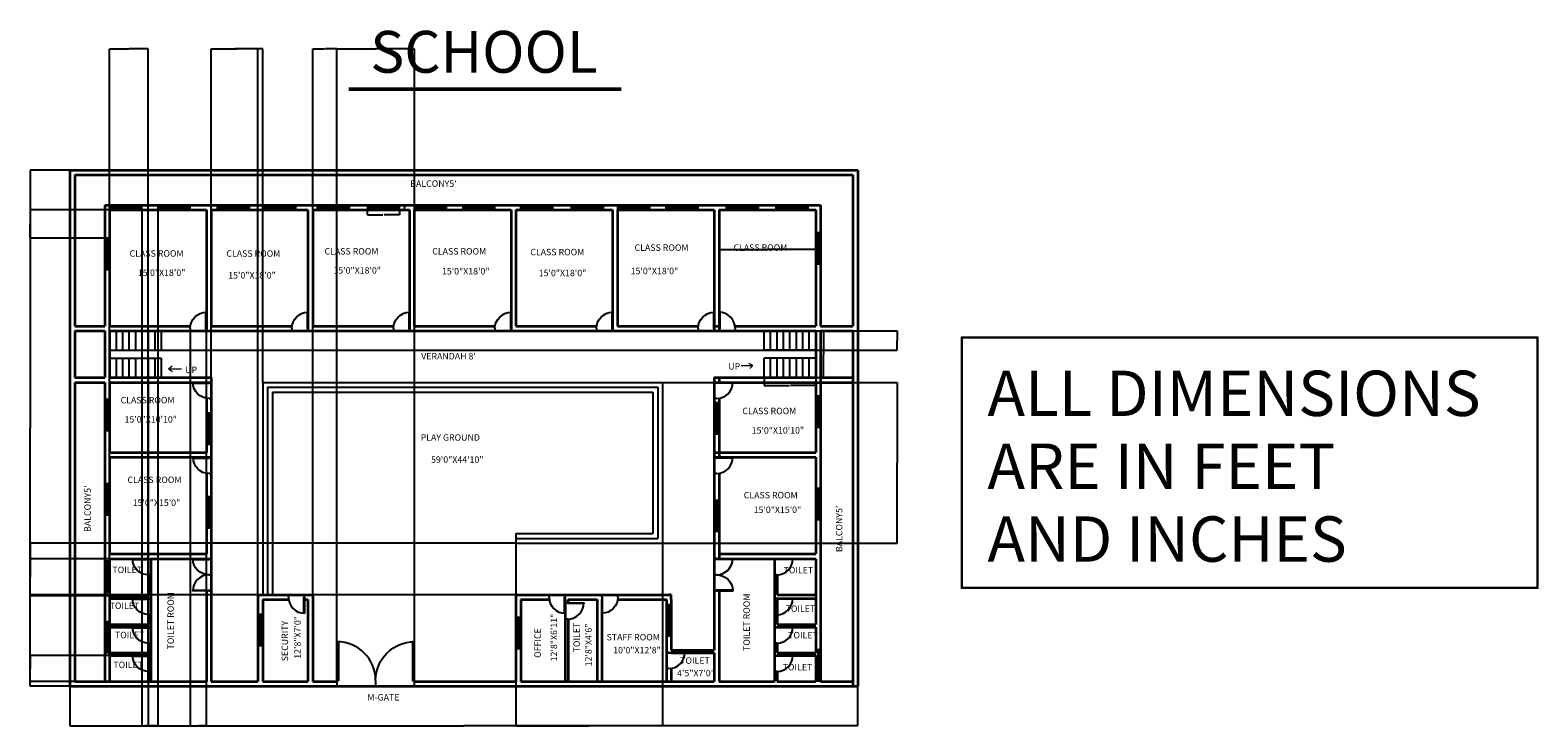
# Model space of a CAD drawing. Units: inches. Extents: x 232314 to 235120, y 482029 to 483323.
import ezdxf

# ---------------------------------------------------------------- set-up
doc = ezdxf.new("R2010")
doc.units = ezdxf.units.IN
for name, color, linetype, lineweight in [('A-ANNO-DIMS', 3, 'Continuous', 18), ('A-ANNO-SYMB', 7, 'Continuous', 18), ('A-ANNO-TEXT', 7, 'Continuous', 18), ('A-ANNO-TTLB', 6, 'Continuous', 35), ('A-AREA-IDEN', 3, 'Continuous', 18), ('A-FLOR-EDGE', 7, 'Continuous', 25), ('A-FLOR-STRS', 7, 'Continuous', 25), ('A-GLAZ', 5, 'Continuous', 18), ('A-WALL', 7, 'Continuous', 35), ('doors', 4, 'Continuous', 25)]:
    doc.layers.add(name, color=color, linetype=linetype, lineweight=lineweight)
doc.styles.get("Standard").update_dxf_attribs({"font": 'arial.ttf'})
doc.dimstyles.get("Standard").update_dxf_attribs({"dimtxt": 0.18, "dimasz": 0.18, "dimexe": 0.18, "dimexo": 0.0625, "dimgap": 0.09, "dimtad": 0, "dimtih": 1, "dimtoh": 1, "dimdec": 4, "dimzin": 0, "dimdsep": 46, "dimtxsty": 'Standard', "dimcen": 0.09, "dimadec": 0, "dimazin": 0, "dimtfac": 1, "dimtdec": 4, "dimtofl": 0, "dimtmove": 0, "dimatfit": 3, "dimfxl": 1, "dimtolj": 1, "dimtzin": 0, "dimarcsym": 0})

# ---------------------------------------------------------------- blocks, each defined once
blk = doc.blocks.new('*U2')
for p, q in [((0, 0), (0, -6)), ((40, 0), (40, -6))]:
    blk.add_line(p, q)
blk.add_lwpolyline([(0, 0), (0, 40), (1.75, 40), (1.75, 0)], close=True)
blk.add_arc((0, 0), 40, 0, 90)
blk = doc.blocks.new('WIN-60X9-IN')
for p, q in [((0, 5.5), (60, 5.5)), ((0, 3.5), (60, 3.5))]:
    blk.add_line(p, q)
blk.add_lwpolyline([(0, 9), (60, 9), (60, 0), (0, 0)], close=True)
blk = doc.blocks.new('STAIR-PAIRED-FLIGHT')
for p, q in [((12, 87), (12, 51)), ((24, 87), (24, 51)), ((36, 87), (36, 51)), ((48, 87), (48, 51)), ((60, 87), (60, 51)), ((72, 87), (72, 51)), ((84, 87), (84, 51)), ((96, 87), (96, 51)), ((0, 51), (96, 51)), ((0, 36), (96, 36)), ((12, 36), (12, 0)), ((24, 36), (24, 0)), ((36, 36), (36, 0)), ((48, 36), (48, 0)), ((60, 36), (60, 0)), ((72, 36), (72, 0)), ((84, 36), (84, 0)), ((96, 36), (96, 0))]:
    blk.add_line(p, q)
blk = doc.blocks.new('*D7')
at = {"layer": 'A-ANNO-DIMS', "color": 0, "lineweight": -2, "transparency": 16777216}
for p, q in [((232941.9, 482988.3), (232941.9, 482979.2)), ((232942.1, 482979.4), (232970.8, 482979.4)), ((233001.7, 482979.4), (232973, 482979.4)), ((233001.9, 482988.3), (233001.9, 482979.2))]:
    blk.add_line(p, q, dxfattribs=at)
at = {"layer": 'A-ANNO-DIMS', "color": 0, "transparency": 16777216}
for points in [[(232942.1, 482979.4), (232942.1, 482979.3), (232941.9, 482979.4)], [(233001.7, 482979.4), (233001.7, 482979.3), (233001.9, 482979.4)]]:
    blk.add_solid(points, dxfattribs=at)
at = {"layer": 'Defpoints', "color": 0, "transparency": 16777216}
for p in [(232941.9, 482988.4), (233001.9, 482988.4), (233001.9, 482979.4)]:
    blk.add_point(p, dxfattribs=at)
at = {"layer": 'A-ANNO-DIMS', "color": 0, "transparency": 16777216, "insert": (232971.9, 482979.4), "char_height": 0.18, "attachment_point": 5}
blk.add_mtext('\\A1;WINDOW 60 TYP.', dxfattribs=at)
blk = doc.blocks.new('*D8')
at = {"layer": 'A-ANNO-DIMS', "color": 0, "lineweight": -2, "transparency": 16777216}
for p, q in [((233002, 482997.4), (233011.1, 482997.4)), ((233002, 482988.4), (233011.1, 482988.4)), ((233010.9, 482997.2), (233010.9, 482993.1)), ((233010.9, 482988.6), (233010.9, 482992.7))]:
    blk.add_line(p, q, dxfattribs=at)
at = {"layer": 'A-ANNO-DIMS', "color": 0, "transparency": 16777216}
for points in [[(233010.9, 482997.2), (233011, 482997.2), (233010.9, 482997.4)], [(233010.9, 482988.6), (233011, 482988.6), (233010.9, 482988.4)]]:
    blk.add_solid(points, dxfattribs=at)
at = {"layer": 'Defpoints', "color": 0, "transparency": 16777216}
for p in [(233001.9, 482997.4), (233001.9, 482988.4), (233010.9, 482997.4)]:
    blk.add_point(p, dxfattribs=at)
at = {"layer": 'A-ANNO-DIMS', "color": 0, "transparency": 16777216, "insert": (233010.9, 482992.9), "char_height": 0.18, "attachment_point": 5}
blk.add_mtext('\\A1;9 TYP.', dxfattribs=at)
blk = doc.blocks.new('*D9')
at = {"layer": 'A-ANNO-DIMS', "color": 0, "lineweight": -2, "transparency": 16777216}
for p, q in [((233680.3, 482676.3), (233680.3, 482661.8)), ((233776.3, 482676.3), (233776.3, 482661.8)), ((233680.5, 482662), (233727.4, 482662)), ((233776.2, 482662), (233729.3, 482662))]:
    blk.add_line(p, q, dxfattribs=at)
at = {"layer": 'A-ANNO-DIMS', "color": 0, "transparency": 16777216}
for points in [[(233680.5, 482662), (233680.5, 482661.9), (233680.3, 482662)], [(233776.2, 482662), (233776.2, 482661.9), (233776.3, 482662)]]:
    blk.add_solid(points, dxfattribs=at)
at = {"layer": 'Defpoints', "color": 0, "transparency": 16777216}
for p in [(233680.3, 482676.4), (233776.3, 482676.4), (233680.3, 482662)]:
    blk.add_point(p, dxfattribs=at)
at = {"layer": 'A-ANNO-DIMS', "color": 0, "transparency": 16777216, "insert": (233728.3, 482662), "char_height": 0.18, "attachment_point": 5}
blk.add_mtext('\\A1;STAIR 96 TYP.', dxfattribs=at)
blk = doc.blocks.new('*D10')
at = {"layer": 'A-ANNO-DIMS', "color": 0, "lineweight": -2, "transparency": 16777216}
for p, q in [((233776.4, 482763.4), (233790.9, 482763.4)), ((233790.7, 482763.2), (233790.7, 482720.1)), ((233790.7, 482676.6), (233790.7, 482719.7)), ((233776.4, 482676.4), (233790.9, 482676.4))]:
    blk.add_line(p, q, dxfattribs=at)
at = {"layer": 'A-ANNO-DIMS', "color": 0, "transparency": 16777216}
for points in [[(233790.7, 482763.2), (233790.8, 482763.2), (233790.7, 482763.4)], [(233790.7, 482676.6), (233790.8, 482676.6), (233790.7, 482676.4)]]:
    blk.add_solid(points, dxfattribs=at)
at = {"layer": 'Defpoints', "color": 0, "transparency": 16777216}
for p in [(233776.3, 482763.4), (233776.3, 482676.4), (233790.7, 482676.4)]:
    blk.add_point(p, dxfattribs=at)
at = {"layer": 'A-ANNO-DIMS', "color": 0, "transparency": 16777216, "insert": (233790.7, 482719.9), "char_height": 0.18, "attachment_point": 5}
blk.add_mtext('\\A1;87 TYP.', dxfattribs=at)
blk = doc.blocks.new('*D11')
at = {"layer": 'A-ANNO-DIMS', "color": 0, "lineweight": -2, "transparency": 16777216}
for p, q in [((232388.3, 482102.3), (232388.3, 482028.6)), ((233854.3, 482102.3), (233854.3, 482028.6)), ((232388.5, 482028.8), (233121, 482028.8)), ((233854.2, 482028.8), (233121.7, 482028.8))]:
    blk.add_line(p, q, dxfattribs=at)
at = {"layer": 'A-ANNO-DIMS', "color": 0, "transparency": 16777216}
for points in [[(232388.5, 482028.9), (232388.5, 482028.8), (232388.3, 482028.8)], [(233854.2, 482028.9), (233854.2, 482028.8), (233854.3, 482028.8)]]:
    blk.add_solid(points, dxfattribs=at)
at = {"layer": 'Defpoints', "color": 0, "transparency": 16777216}
for p in [(232388.3, 482102.4), (233854.3, 482102.4), (233854.3, 482028.8)]:
    blk.add_point(p, dxfattribs=at)
at = {"layer": 'A-ANNO-DIMS', "color": 0, "transparency": 16777216, "insert": (233121.3, 482028.8), "char_height": 0.18, "attachment_point": 5}
blk.add_mtext('\\A1;1466', dxfattribs=at)
blk = doc.blocks.new('*D12')
at = {"layer": 'A-ANNO-DIMS', "color": 0, "lineweight": -2, "transparency": 16777216}
for p, q in [((232388.3, 483062.4), (232314.6, 483062.4)), ((232314.8, 483062.2), (232314.8, 482582.6)), ((232314.8, 482102.6), (232314.8, 482582.2)), ((232388.3, 482102.4), (232314.6, 482102.4))]:
    blk.add_line(p, q, dxfattribs=at)
at = {"layer": 'A-ANNO-DIMS', "color": 0, "transparency": 16777216}
for points in [[(232314.8, 483062.2), (232314.8, 483062.2), (232314.8, 483062.4)], [(232314.8, 482102.6), (232314.8, 482102.6), (232314.8, 482102.4)]]:
    blk.add_solid(points, dxfattribs=at)
at = {"layer": 'Defpoints', "color": 0, "transparency": 16777216}
for p in [(232314.8, 483062.4), (232388.3, 483062.4), (232388.3, 482102.4)]:
    blk.add_point(p, dxfattribs=at)
at = {"layer": 'A-ANNO-DIMS', "color": 0, "transparency": 16777216, "insert": (232314.8, 482582.4), "char_height": 0.18, "attachment_point": 5}
blk.add_mtext('\\A1;960', dxfattribs=at)
blk = doc.blocks.new('*D13')
at = {"layer": 'A-ANNO-DIMS', "color": 0, "lineweight": -2, "transparency": 16777216}
for p, q in [((232840.3, 482111.4), (232840.3, 483288)), ((232840.5, 483287.8), (232862.4, 483287.8)), ((232885.2, 483287.8), (232863.2, 483287.8)), ((232885.4, 482111.4), (232885.4, 483288))]:
    blk.add_line(p, q, dxfattribs=at)
at = {"layer": 'A-ANNO-DIMS', "color": 0, "transparency": 16777216}
for points in [[(232840.5, 483287.9), (232840.5, 483287.8), (232840.3, 483287.8)], [(232885.2, 483287.9), (232885.2, 483287.8), (232885.4, 483287.8)]]:
    blk.add_solid(points, dxfattribs=at)
at = {"layer": 'Defpoints', "color": 0, "transparency": 16777216}
for p in [(232885.4, 483287.8), (232840.3, 482111.4), (232885.4, 482111.4)]:
    blk.add_point(p, dxfattribs=at)
at = {"layer": 'A-ANNO-DIMS', "color": 0, "transparency": 16777216, "insert": (232862.8, 483287.8), "char_height": 0.18, "attachment_point": 5}
blk.add_mtext('\\A1;45.02', dxfattribs=at)
blk = doc.blocks.new('*D14')
at = {"layer": 'A-ANNO-DIMS', "color": 0, "lineweight": -2, "transparency": 16777216}
for p, q in [((232885.4, 482111.4), (232885.4, 483288)), ((232885.5, 483287.8), (232957.1, 483287.8)), ((233029.2, 483287.8), (232957.6, 483287.8)), ((233029.4, 482111.4), (233029.4, 483288))]:
    blk.add_line(p, q, dxfattribs=at)
at = {"layer": 'A-ANNO-DIMS', "color": 0, "transparency": 16777216}
for points in [[(232885.5, 483287.9), (232885.5, 483287.8), (232885.4, 483287.8)], [(233029.2, 483287.9), (233029.2, 483287.8), (233029.4, 483287.8)]]:
    blk.add_solid(points, dxfattribs=at)
at = {"layer": 'Defpoints', "color": 0, "transparency": 16777216}
for p in [(233029.4, 483287.8), (232885.4, 482111.4), (233029.4, 482111.4)]:
    blk.add_point(p, dxfattribs=at)
at = {"layer": 'A-ANNO-DIMS', "color": 0, "transparency": 16777216, "insert": (232957.4, 483287.8), "char_height": 0.18, "attachment_point": 5}
blk.add_mtext('\\A1;144', dxfattribs=at)
blk = doc.blocks.new('*D15')
at = {"layer": 'A-ANNO-DIMS', "color": 0, "lineweight": -2, "transparency": 16777216}
for p, q in [((232612.2, 482763.3), (232612.2, 482028.6)), ((232642.3, 482763.3), (232642.3, 482028.6)), ((232612.4, 482028.8), (232626.9, 482028.8)), ((232642.2, 482028.8), (232627.7, 482028.8))]:
    blk.add_line(p, q, dxfattribs=at)
at = {"layer": 'A-ANNO-DIMS', "color": 0, "transparency": 16777216}
for points in [[(232612.4, 482028.9), (232612.4, 482028.8), (232612.2, 482028.8)], [(232642.2, 482028.9), (232642.2, 482028.8), (232642.3, 482028.8)]]:
    blk.add_solid(points, dxfattribs=at)
at = {"layer": 'Defpoints', "color": 0, "transparency": 16777216}
for p in [(232612.2, 482763.4), (232642.3, 482763.4), (232642.3, 482028.8)]:
    blk.add_point(p, dxfattribs=at)
at = {"layer": 'A-ANNO-DIMS', "color": 0, "transparency": 16777216, "insert": (232627.3, 482028.8), "char_height": 0.18, "attachment_point": 5}
blk.add_mtext('\\A1;30.09', dxfattribs=at)
blk = doc.blocks.new('*D16')
at = {"layer": 'A-ANNO-DIMS', "color": 0, "lineweight": -2, "transparency": 16777216}
for p, q in [((232651.3, 482111.4), (232651.3, 483288)), ((232651.5, 483287.8), (232694.6, 483287.8)), ((232738.2, 483287.8), (232695.1, 483287.8)), ((232738.3, 482111.4), (232738.3, 483288))]:
    blk.add_line(p, q, dxfattribs=at)
at = {"layer": 'A-ANNO-DIMS', "color": 0, "transparency": 16777216}
for points in [[(232651.5, 483287.9), (232651.5, 483287.8), (232651.3, 483287.8)], [(232738.2, 483287.9), (232738.2, 483287.8), (232738.3, 483287.8)]]:
    blk.add_solid(points, dxfattribs=at)
at = {"layer": 'Defpoints', "color": 0, "transparency": 16777216}
for p in [(232738.3, 483287.8), (232651.3, 482111.4), (232738.3, 482111.4)]:
    blk.add_point(p, dxfattribs=at)
at = {"layer": 'A-ANNO-DIMS', "color": 0, "transparency": 16777216, "insert": (232694.8, 483287.8), "char_height": 0.18, "attachment_point": 5}
blk.add_mtext('\\A1;87', dxfattribs=at)
blk = doc.blocks.new('*D17')
at = {"layer": 'A-ANNO-DIMS', "color": 0, "lineweight": -2, "transparency": 16777216}
for p, q in [((232462.3, 482111.4), (232462.3, 483288)), ((232462.5, 483287.8), (232498.1, 483287.8)), ((232534.2, 483287.8), (232498.5, 483287.8)), ((232534.3, 482111.4), (232534.3, 483288))]:
    blk.add_line(p, q, dxfattribs=at)
at = {"layer": 'A-ANNO-DIMS', "color": 0, "transparency": 16777216}
for points in [[(232462.5, 483287.9), (232462.5, 483287.8), (232462.3, 483287.8)], [(232534.2, 483287.9), (232534.2, 483287.8), (232534.3, 483287.8)]]:
    blk.add_solid(points, dxfattribs=at)
at = {"layer": 'Defpoints', "color": 0, "transparency": 16777216}
for p in [(232534.3, 483287.8), (232462.3, 482111.4), (232534.3, 482111.4)]:
    blk.add_point(p, dxfattribs=at)
at = {"layer": 'A-ANNO-DIMS', "color": 0, "transparency": 16777216, "insert": (232498.3, 483287.8), "char_height": 0.18, "attachment_point": 5}
blk.add_mtext('\\A1;72', dxfattribs=at)
blk = doc.blocks.new('*D18')
at = {"layer": 'A-ANNO-DIMS', "color": 0, "lineweight": -2, "transparency": 16777216}
for p, q in [((232462.3, 482159.4), (232314.6, 482159.4)), ((232314.8, 482159.2), (232314.8, 482135.6)), ((232314.8, 482111.6), (232314.8, 482135.2)), ((232462.3, 482111.4), (232314.6, 482111.4))]:
    blk.add_line(p, q, dxfattribs=at)
at = {"layer": 'A-ANNO-DIMS', "color": 0, "transparency": 16777216}
for points in [[(232314.8, 482159.2), (232314.8, 482159.2), (232314.8, 482159.4)], [(232314.8, 482111.6), (232314.8, 482111.6), (232314.8, 482111.4)]]:
    blk.add_solid(points, dxfattribs=at)
at = {"layer": 'Defpoints', "color": 0, "transparency": 16777216}
for p in [(232314.8, 482159.4), (232462.3, 482159.4), (232462.3, 482111.4)]:
    blk.add_point(p, dxfattribs=at)
at = {"layer": 'A-ANNO-DIMS', "color": 0, "transparency": 16777216, "insert": (232314.8, 482135.4), "char_height": 0.18, "attachment_point": 5}
blk.add_mtext('\\A1;48', dxfattribs=at)
blk = doc.blocks.new('*D19')
at = {"layer": 'A-ANNO-DIMS', "color": 0, "lineweight": -2, "transparency": 16777216}
for p, q in [((232462.3, 482339.4), (232314.6, 482339.4)), ((232314.8, 482339.2), (232314.8, 482305.1)), ((232314.8, 482270.6), (232314.8, 482304.7)), ((232462.3, 482270.4), (232314.6, 482270.4))]:
    blk.add_line(p, q, dxfattribs=at)
at = {"layer": 'A-ANNO-DIMS', "color": 0, "transparency": 16777216}
for points in [[(232314.8, 482339.2), (232314.8, 482339.2), (232314.8, 482339.4)], [(232314.8, 482270.6), (232314.8, 482270.6), (232314.8, 482270.4)]]:
    blk.add_solid(points, dxfattribs=at)
at = {"layer": 'Defpoints', "color": 0, "transparency": 16777216}
for p in [(232314.8, 482339.4), (232462.3, 482339.4), (232462.3, 482270.4)]:
    blk.add_point(p, dxfattribs=at)
at = {"layer": 'A-ANNO-DIMS', "color": 0, "transparency": 16777216, "insert": (232314.8, 482304.9), "char_height": 0.18, "attachment_point": 5}
blk.add_mtext('\\A1;69', dxfattribs=at)
blk = doc.blocks.new('*D20')
at = {"layer": 'A-ANNO-DIMS', "color": 0, "lineweight": -2, "transparency": 16777216}
for p, q in [((232522.3, 482988.3), (232522.3, 482028.6)), ((232552.3, 482988.3), (232552.3, 482028.6)), ((232522.5, 482028.8), (232537.1, 482028.8)), ((232552.2, 482028.8), (232537.5, 482028.8))]:
    blk.add_line(p, q, dxfattribs=at)
at = {"layer": 'A-ANNO-DIMS', "color": 0, "transparency": 16777216}
for points in [[(232522.5, 482028.9), (232522.5, 482028.8), (232522.3, 482028.8)], [(232552.2, 482028.9), (232552.2, 482028.8), (232552.3, 482028.8)]]:
    blk.add_solid(points, dxfattribs=at)
at = {"layer": 'Defpoints', "color": 0, "transparency": 16777216}
for p in [(232522.3, 482988.4), (232552.3, 482988.4), (232552.3, 482028.8)]:
    blk.add_point(p, dxfattribs=at)
at = {"layer": 'A-ANNO-DIMS', "color": 0, "transparency": 16777216, "insert": (232537.3, 482028.8), "char_height": 0.18, "attachment_point": 5}
blk.add_mtext('\\A1;30', dxfattribs=at)
blk = doc.blocks.new('*D21')
at = {"layer": 'A-ANNO-DIMS', "color": 0, "lineweight": -2, "transparency": 16777216}
for p, q in [((232462.3, 482988.4), (232314.6, 482988.4)), ((232314.8, 482988.2), (232314.8, 482962.4)), ((232314.8, 482936.2), (232314.8, 482962)), ((232462.3, 482936), (232314.6, 482936))]:
    blk.add_line(p, q, dxfattribs=at)
at = {"layer": 'A-ANNO-DIMS', "color": 0, "transparency": 16777216}
for points in [[(232314.8, 482988.2), (232314.8, 482988.2), (232314.8, 482988.4)], [(232314.8, 482936.2), (232314.8, 482936.2), (232314.8, 482936)]]:
    blk.add_solid(points, dxfattribs=at)
at = {"layer": 'Defpoints', "color": 0, "transparency": 16777216}
for p in [(232314.8, 482988.4), (232462.3, 482988.4), (232462.3, 482936)]:
    blk.add_point(p, dxfattribs=at)
at = {"layer": 'A-ANNO-DIMS', "color": 0, "transparency": 16777216, "insert": (232314.8, 482962.2), "char_height": 0.18, "attachment_point": 5}
blk.add_mtext('\\A1;52.34', dxfattribs=at)
blk = doc.blocks.new('*D22')
at = {"layer": 'A-ANNO-DIMS', "color": 0, "lineweight": -2, "transparency": 16777216}
for p, q in [((232651.3, 482667.4), (232651.3, 483288)), ((232651.5, 483287.8), (232699.1, 483287.8)), ((232747.2, 483287.8), (232699.5, 483287.8)), ((232747.3, 482667.4), (232747.3, 483288))]:
    blk.add_line(p, q, dxfattribs=at)
at = {"layer": 'A-ANNO-DIMS', "color": 0, "transparency": 16777216}
for points in [[(232651.5, 483287.9), (232651.5, 483287.8), (232651.3, 483287.8)], [(232747.2, 483287.9), (232747.2, 483287.8), (232747.3, 483287.8)]]:
    blk.add_solid(points, dxfattribs=at)
at = {"layer": 'Defpoints', "color": 0, "transparency": 16777216}
for p in [(232747.3, 483287.8), (232651.3, 482667.4), (232747.3, 482667.4)]:
    blk.add_point(p, dxfattribs=at)
at = {"layer": 'A-ANNO-DIMS', "color": 0, "transparency": 16777216, "insert": (232699.3, 483287.8), "char_height": 0.18, "attachment_point": 5}
blk.add_mtext('\\A1;96', dxfattribs=at)
blk = doc.blocks.new('*D23')
at = {"layer": 'A-ANNO-DIMS', "color": 0, "lineweight": -2, "transparency": 16777216}
for p, q in [((233218.330976, 482368.308229), (233218.330976, 482028.640729)), ((233491.330976, 482368.308229), (233491.330976, 482028.640729)), ((233218.510976, 482028.820729), (233354.540594, 482028.820729)), ((233491.150976, 482028.820729), (233355.121358, 482028.820729))]:
    blk.add_line(p, q, dxfattribs=at)
at = {"layer": 'A-ANNO-DIMS', "color": 0, "transparency": 16777216}
for points in [[(233218.510976, 482028.850729), (233218.510976, 482028.790729), (233218.330976, 482028.820729)], [(233491.150976, 482028.850729), (233491.150976, 482028.790729), (233491.330976, 482028.820729)]]:
    blk.add_solid(points, dxfattribs=at)
at = {"layer": 'Defpoints', "color": 0, "transparency": 16777216}
for p in [(233218.330976, 482368.370729), (233491.330976, 482368.370729), (233218.330976, 482028.820729)]:
    blk.add_point(p, dxfattribs=at)
at = {"layer": 'A-ANNO-DIMS', "color": 0, "transparency": 16777216, "insert": (233354.830976, 482028.820729), "char_height": 0.18, "attachment_point": 5}
blk.add_mtext('\\A1;273', dxfattribs=at)
blk = doc.blocks.new('*D24')
at = {"layer": 'A-ANNO-DIMS', "color": 0, "lineweight": -2, "transparency": 16777216}
for p, q in [((233218.3, 482368.4), (232314.6, 482368.4)), ((232314.8, 482368.2), (232314.8, 482320.6)), ((232314.8, 482272.6), (232314.8, 482320.2)), ((233218.3, 482272.4), (232314.6, 482272.4))]:
    blk.add_line(p, q, dxfattribs=at)
at = {"layer": 'A-ANNO-DIMS', "color": 0, "transparency": 16777216}
for points in [[(232314.8, 482368.2), (232314.8, 482368.2), (232314.8, 482368.4)], [(232314.8, 482272.6), (232314.8, 482272.6), (232314.8, 482272.4)]]:
    blk.add_solid(points, dxfattribs=at)
at = {"layer": 'Defpoints', "color": 0, "transparency": 16777216}
for p in [(233218.3, 482368.4), (232314.8, 482272.4), (233218.3, 482272.4)]:
    blk.add_point(p, dxfattribs=at)
at = {"layer": 'A-ANNO-DIMS', "color": 0, "transparency": 16777216, "insert": (232314.8, 482320.4), "char_height": 0.18, "attachment_point": 5}
blk.add_mtext('\\A1;96', dxfattribs=at)
blk = doc.blocks.new('*D25')
at = {"layer": 'A-ANNO-DIMS', "color": 0, "lineweight": -2, "transparency": 16777216}
for p, q in [((233491.4, 482667.4), (233928.1, 482667.4)), ((233927.9, 482667.2), (233927.9, 482518.1)), ((233927.9, 482368.6), (233927.9, 482517.7)), ((233491.4, 482368.4), (233928.1, 482368.4))]:
    blk.add_line(p, q, dxfattribs=at)
at = {"layer": 'A-ANNO-DIMS', "color": 0, "transparency": 16777216}
for points in [[(233927.9, 482667.2), (233927.9, 482667.2), (233927.9, 482667.4)], [(233927.9, 482368.6), (233927.9, 482368.6), (233927.9, 482368.4)]]:
    blk.add_solid(points, dxfattribs=at)
at = {"layer": 'Defpoints', "color": 0, "transparency": 16777216}
for p in [(233491.3, 482667.4), (233491.3, 482368.4), (233927.9, 482368.4)]:
    blk.add_point(p, dxfattribs=at)
at = {"layer": 'A-ANNO-DIMS', "color": 0, "transparency": 16777216, "insert": (233927.9, 482517.9), "char_height": 0.18, "attachment_point": 5}
blk.add_mtext('\\A1;299', dxfattribs=at)
blk = doc.blocks.new('*D26')
at = {"layer": 'A-ANNO-DIMS', "color": 0, "lineweight": -2, "transparency": 16777216}
for p, q in [((233596.3, 482988.3), (233596.3, 482914.6)), ((233776.3, 482988.3), (233776.3, 482914.6)), ((233596.5, 482914.8), (233686.1, 482914.8)), ((233776.2, 482914.8), (233686.6, 482914.8))]:
    blk.add_line(p, q, dxfattribs=at)
at = {"layer": 'A-ANNO-DIMS', "color": 0, "transparency": 16777216}
for points in [[(233596.5, 482914.9), (233596.5, 482914.8), (233596.3, 482914.8)], [(233776.2, 482914.9), (233776.2, 482914.8), (233776.3, 482914.8)]]:
    blk.add_solid(points, dxfattribs=at)
at = {"layer": 'Defpoints', "color": 0, "transparency": 16777216}
for p in [(233596.3, 482988.4), (233776.3, 482988.4), (233596.3, 482914.8)]:
    blk.add_point(p, dxfattribs=at)
at = {"layer": 'A-ANNO-DIMS', "color": 0, "transparency": 16777216, "insert": (233686.3, 482914.8), "char_height": 0.18, "attachment_point": 5}
blk.add_mtext('\\A1;180', dxfattribs=at)
blk = doc.blocks.new('*D27')
at = {"layer": 'A-ANNO-DIMS', "color": 0, "lineweight": -2, "transparency": 16777216}
for p, q in [((232558.4, 482763.4), (233928.1, 482763.4)), ((233927.9, 482763.2), (233927.9, 482745.6)), ((232558.4, 482727.4), (233928.1, 482727.4)), ((233927.9, 482727.6), (233927.9, 482745.2))]:
    blk.add_line(p, q, dxfattribs=at)
at = {"layer": 'A-ANNO-DIMS', "color": 0, "transparency": 16777216}
for points in [[(233927.9, 482763.2), (233927.9, 482763.2), (233927.9, 482763.4)], [(233927.9, 482727.6), (233927.9, 482727.6), (233927.9, 482727.4)]]:
    blk.add_solid(points, dxfattribs=at)
at = {"layer": 'Defpoints', "color": 0, "transparency": 16777216}
for p in [(232558.3, 482763.4), (232558.3, 482727.4), (233927.9, 482727.4)]:
    blk.add_point(p, dxfattribs=at)
at = {"layer": 'A-ANNO-DIMS', "color": 0, "transparency": 16777216, "insert": (233927.9, 482745.4), "char_height": 0.18, "attachment_point": 5}
blk.add_mtext('\\A1;36', dxfattribs=at)
blk = doc.blocks.new('*D28')
at = {"layer": 'A-ANNO-DIMS', "color": 0, "lineweight": -2, "transparency": 16777216}
for p, q in [((232522.3, 482676.3), (232522.3, 482028.6)), ((232534.3, 482676.3), (232534.3, 482028.6)), ((232522.5, 482028.8), (232528.1, 482028.8)), ((232534.2, 482028.8), (232528.5, 482028.8))]:
    blk.add_line(p, q, dxfattribs=at)
at = {"layer": 'A-ANNO-DIMS', "color": 0, "transparency": 16777216}
for points in [[(232522.5, 482028.9), (232522.5, 482028.8), (232522.3, 482028.8)], [(232534.2, 482028.9), (232534.2, 482028.8), (232534.3, 482028.8)]]:
    blk.add_solid(points, dxfattribs=at)
at = {"layer": 'Defpoints', "color": 0, "transparency": 16777216}
for p in [(232522.3, 482676.4), (232534.3, 482676.4), (232534.3, 482028.8)]:
    blk.add_point(p, dxfattribs=at)
at = {"layer": 'A-ANNO-DIMS', "color": 0, "transparency": 16777216, "insert": (232528.3, 482028.8), "char_height": 0.18, "attachment_point": 5}
blk.add_mtext('\\A1;12', dxfattribs=at)

msp = doc.modelspace()

# ---------------------------------------------------------------- linework, layer by layer
at = {"layer": 'A-ANNO-SYMB'}
for p, q in [((232572.017, 482692.814), (232578.651, 482698.51)), ((232572.017, 482692.814), (232596.272, 482692.814)), ((232572.017, 482692.814), (232579.273, 482687.739)), ((233637.386, 482698.759), (233659.472, 482698.759)), ((233659.472, 482698.759), (233651.752, 482702.585)), ((233659.472, 482698.759), (233653.688, 482693.504))]:
    msp.add_line(p, q, dxfattribs=at)
at = {"layer": 'A-ANNO-TEXT'}
for points in [[(234047.316, 482752.496), (235120.006, 482752.496), (235120.006, 482283.952), (234047.316, 482283.952)], [(234049.316, 482750.496), (235118.006, 482750.496), (235118.006, 482285.952), (234049.316, 482285.952)]]:
    msp.add_lwpolyline(points, close=True, dxfattribs=at)
at = {"layer": 'A-ANNO-TTLB'}
for p, q in [((232907.501, 483214.294), (233414.412, 483214.294)), ((232907.501, 483212.294), (233414.412, 483212.294))]:
    msp.add_line(p, q, dxfattribs=at)
at = {"layer": 'A-FLOR-EDGE'}
for p, q in [((232747.331, 482667.371), (232747.331, 482272.371)), ((232747.331, 482667.371), (233491.331, 482667.371)), ((233491.331, 482667.371), (233491.331, 482368.371)), ((232756.331, 482658.371), (232756.331, 482272.371)), ((232756.331, 482658.371), (233482.331, 482658.371)), ((232765.331, 482649.371), (232765.331, 482272.371)), ((232765.331, 482649.371), (233473.331, 482649.371)), ((233473.331, 482649.371), (233473.331, 482386.371)), ((233482.331, 482658.371), (233482.331, 482377.371)), ((233218.331, 482386.371), (233473.331, 482386.371)), ((233218.331, 482386.371), (233218.331, 482368.371)), ((233218.331, 482377.371), (233482.331, 482377.371)), ((233218.331, 482368.371), (233491.331, 482368.371))]:
    msp.add_line(p, q, dxfattribs=at)
at = {"layer": 'A-WALL'}
for p, q in [((232388.331, 483062.371), (233854.331, 483062.371)), ((232388.331, 483062.371), (232388.331, 482102.371)), ((233854.331, 483062.371), (233854.331, 482102.371)), ((232397.331, 483053.371), (233845.331, 483053.371)), ((232397.331, 483053.371), (232397.331, 482993.371)), ((232397.331, 483053.371), (232397.331, 482772.371)), ((233845.331, 483053.371), (233845.331, 482772.371)), ((232453.331, 482997.371), (233785.331, 482997.371)), ((232453.331, 482997.371), (232453.331, 482772.371)), ((232462.331, 482988.371), (232642.331, 482988.371)), ((232462.331, 482988.371), (232462.331, 482772.371)), ((232642.331, 482988.371), (232642.331, 482763.371)), ((232651.331, 482988.371), (232651.331, 482772.371)), ((232651.331, 482988.371), (232831.331, 482988.371)), ((232831.331, 482988.371), (232831.331, 482763.371)), ((232840.331, 482988.371), (232840.331, 482772.371)), ((232840.331, 482988.371), (233020.331, 482988.371)), ((233020.331, 482988.371), (233020.331, 482763.371)), ((233029.331, 482988.371), (233029.331, 482772.371)), ((233029.331, 482988.371), (233209.331, 482988.371)), ((233209.331, 482988.371), (233209.331, 482763.371)), ((233218.331, 482988.371), (233218.331, 482772.371)), ((233218.331, 482988.371), (233398.331, 482988.371)), ((233398.331, 482988.371), (233398.331, 482763.371)), ((233407.331, 482988.371), (233407.331, 482772.371)), ((233407.331, 482988.371), (233587.331, 482988.371)), ((233587.331, 482988.371), (233587.331, 482763.371)), ((233596.331, 482988.371), (233596.331, 482763.371)), ((233596.331, 482988.371), (233776.331, 482988.371)), ((233776.331, 482988.371), (233776.331, 482772.371)), ((233785.331, 482997.371), (233785.331, 482772.371)), ((232397.331, 482772.371), (232453.331, 482772.371)), ((232397.331, 482763.371), (232453.331, 482763.371)), ((232397.331, 482763.371), (232397.331, 482676.371)), ((232453.331, 482763.371), (232453.331, 482676.371)), ((232462.331, 482772.371), (232612.582, 482772.371)), ((232462.331, 482763.371), (232462.331, 482676.371)), ((232462.331, 482763.371), (233776.331, 482763.371)), ((232640.93, 482772.371), (232642.331, 482772.371)), ((232651.331, 482772.371), (232801.641, 482772.371)), ((232829.989, 482772.371), (232831.331, 482772.371)), ((232840.331, 482772.371), (232990.733, 482772.371)), ((233019.081, 482772.371), (233020.394, 482772.371)), ((233029.331, 482772.371), (233179.733, 482772.371)), ((233208.081, 482772.371), (233209.394, 482772.371)), ((233218.331, 482772.371), (233368.446, 482772.371)), ((233396.794, 482772.371), (233398.331, 482772.371)), ((233407.331, 482772.371), (233557.663, 482772.371)), ((233586.011, 482772.371), (233597.643, 482772.371)), ((233625.992, 482772.371), (233776.331, 482772.371)), ((233776.331, 482763.371), (233776.331, 482727.371)), ((233785.331, 482772.371), (233845.331, 482772.371)), ((233785.331, 482763.371), (233785.331, 482727.371)), ((233785.331, 482763.371), (233845.331, 482763.371)), ((233845.331, 482763.371), (233845.331, 482102.371)), ((233776.331, 482727.371), (233776.331, 482676.371)), ((233785.331, 482727.371), (233785.331, 482111.371)), ((232397.331, 482676.371), (232453.331, 482676.371)), ((232397.331, 482667.371), (232453.331, 482667.371)), ((232397.331, 482667.371), (232397.331, 482111.371)), ((232453.331, 482667.371), (232453.331, 482111.371)), ((232462.331, 482676.371), (232642.331, 482676.371)), ((232462.331, 482667.371), (232462.331, 482537.371)), ((232462.331, 482667.371), (232642.331, 482667.371)), ((232642.331, 482676.371), (232651.331, 482676.371)), ((232642.331, 482667.526), (232642.331, 482666.213)), ((232642.331, 482667.371), (232651.331, 482667.371)), ((232651.331, 482676.371), (232651.331, 482667.526)), ((232651.331, 482667.526), (232651.331, 482111.371)), ((233587.331, 482676.371), (233776.331, 482676.371)), ((233587.331, 482676.371), (233587.331, 482272.371)), ((233587.331, 482667.371), (233845.331, 482667.371)), ((233596.331, 482676.371), (233596.331, 482666.188)), ((233776.331, 482667.371), (233776.331, 482537.371)), ((233785.331, 482676.371), (233845.331, 482676.371)), ((232642.331, 482637.948), (232642.331, 482537.371)), ((233596.331, 482637.84), (233596.331, 482526.819)), ((232462.331, 482537.371), (232642.331, 482537.371)), ((232462.331, 482528.371), (232651.331, 482528.371)), ((232462.331, 482528.371), (232462.331, 482348.371)), ((232642.331, 482528.371), (232642.331, 482526.441)), ((233587.331, 482537.371), (233776.331, 482537.371)), ((233587.331, 482528.371), (233776.331, 482528.371)), ((233776.331, 482528.371), (233776.331, 482348.371)), ((232642.331, 482498.225), (232642.331, 482348.371)), ((233596.331, 482498.471), (233596.331, 482338.382)), ((232462.331, 482348.371), (232642.331, 482348.371)), ((232462.331, 482339.371), (232534.331, 482339.371)), ((232462.331, 482339.371), (232462.331, 482111.371)), ((232534.331, 482339.371), (232534.331, 482337.995)), ((232539.331, 482339.371), (232539.331, 482111.371)), ((232539.331, 482339.371), (232651.331, 482339.371)), ((232642.331, 482339.371), (232642.331, 482338.054)), ((233587.331, 482339.371), (233776.331, 482339.371)), ((233596.331, 482348.371), (233776.331, 482348.371)), ((233699.331, 482339.41), (233699.331, 482212.371)), ((233704.331, 482339.41), (233704.331, 482338.098)), ((233776.331, 482339.371), (233776.331, 482265.371)), ((232534.331, 482309.315), (232534.331, 482270.371)), ((232642.331, 482309.783), (232642.331, 482309.402)), ((233596.331, 482310.034), (233596.331, 482309.355)), ((233704.331, 482309.414), (233704.331, 482272.371)), ((232642.331, 482281.13), (232642.331, 482111.371)), ((232738.331, 482272.371), (232840.331, 482272.371)), ((232738.331, 482272.371), (232738.331, 482111.371)), ((232840.331, 482272.371), (232840.331, 482111.371)), ((233218.331, 482272.371), (233218.331, 482111.371)), ((233218.331, 482272.371), (233503.331, 482272.371)), ((233507.331, 482272.371), (233503.331, 482272.371)), ((233507.331, 482263.371), (233507.331, 482272.371)), ((233587.331, 482279.695), (233587.331, 482169.371)), ((233596.331, 482281.007), (233596.331, 482263.371)), ((233704.331, 482272.371), (233776.331, 482272.371)), ((232462.331, 482270.371), (232534.331, 482270.371)), ((232462.331, 482265.371), (232539.331, 482265.371)), ((232534.331, 482265.582), (232534.331, 482264.269)), ((232747.331, 482263.371), (232795.509, 482263.371)), ((232747.331, 482263.371), (232747.331, 482111.371)), ((232823.844, 482263.371), (232831.331, 482263.371)), ((232831.331, 482263.371), (232831.331, 482111.371)), ((233227.331, 482263.371), (233227.331, 482111.371)), ((233227.331, 482263.371), (233280.422, 482263.371)), ((233308.757, 482263.371), (233310.331, 482263.371)), ((233310.331, 482263.371), (233310.331, 482111.371)), ((233315.331, 482263.371), (233315.331, 482256.017)), ((233315.331, 482263.371), (233369.331, 482263.371)), ((233369.331, 482263.371), (233369.331, 482111.371)), ((233378.331, 482263.371), (233378.331, 482111.371)), ((233378.331, 482263.371), (233379.643, 482263.371)), ((233407.978, 482263.371), (233498.331, 482263.371)), ((233498.331, 482263.603), (233498.331, 482263.371)), ((233498.331, 482263.371), (233498.331, 482111.371)), ((233507.331, 482263.371), (233507.331, 482169.371)), ((233596.331, 482265.371), (233596.331, 482262.29)), ((233596.331, 482263.371), (233596.331, 482111.371)), ((233699.331, 482265.371), (233776.331, 482265.371)), ((233704.331, 482265.415), (233704.331, 482217.371)), ((233704.331, 482265.371), (233704.331, 482264.102)), ((233776.331, 482265.371), (233776.331, 482217.371)), ((232462.331, 482217.371), (232534.331, 482217.371)), ((232534.331, 482235.583), (232534.331, 482217.371)), ((233315.331, 482227.334), (233315.331, 482111.371)), ((233596.331, 482233.942), (233596.331, 482233.263)), ((233704.331, 482235.419), (233704.331, 482217.371)), ((233704.331, 482217.371), (233776.331, 482217.371)), ((232462.331, 482212.371), (232539.331, 482212.371)), ((232534.331, 482212.463), (232534.331, 482211.151)), ((233699.331, 482212.371), (233699.331, 482159.371)), ((233699.331, 482212.371), (233776.331, 482212.371)), ((233704.331, 482212.371), (233704.331, 482211.032)), ((233776.331, 482212.371), (233776.331, 482164.371)), ((232462.331, 482164.371), (232534.331, 482164.371)), ((232462.331, 482159.371), (232534.848, 482159.371)), ((232534.331, 482182.467), (232534.331, 482111.371)), ((233507.331, 482169.371), (233587.331, 482169.371)), ((233507.331, 482164.371), (233587.331, 482164.371)), ((233507.331, 482164.371), (233507.331, 482163.778)), ((233587.331, 482164.371), (233587.331, 482111.371)), ((233699.331, 482159.371), (233699.331, 482111.371)), ((233699.331, 482159.371), (233776.331, 482159.371)), ((233704.331, 482182.348), (233704.331, 482164.371)), ((233704.331, 482164.371), (233776.331, 482164.371)), ((233704.331, 482159.371), (233704.331, 482158.29)), ((233776.331, 482159.371), (233776.331, 482111.371)), ((233507.331, 482135.43), (233507.331, 482111.371)), ((232397.331, 482111.371), (232462.331, 482111.371)), ((232462.331, 482111.371), (232642.331, 482111.371)), ((232651.331, 482111.371), (232738.331, 482111.371)), ((232747.331, 482111.371), (232831.331, 482111.371)), ((232840.331, 482111.371), (232885.355, 482111.371)), ((233029.355, 482111.371), (233218.331, 482111.371)), ((233227.331, 482111.371), (233498.331, 482111.371)), ((233498.331, 482111.371), (233587.331, 482111.371)), ((233596.331, 482111.371), (233699.331, 482111.371)), ((233704.331, 482129.607), (233704.331, 482111.371)), ((233704.331, 482111.371), (233776.331, 482111.371)), ((233785.331, 482111.371), (233845.331, 482111.371)), ((232388.331, 482102.371), (233854.331, 482102.371))]:
    msp.add_line(p, q, dxfattribs=at)

# ---------------------------------------------------------------- block references
at = {"layer": 'A-FLOR-STRS'}
msp.add_blockref('STAIR-PAIRED-FLIGHT', (232462.331, 482676.371), dxfattribs=at)
at = {"layer": 'A-FLOR-STRS', "rotation": 180}
msp.add_blockref('STAIR-PAIRED-FLIGHT', (233776.331, 482763.371), dxfattribs=at)
at = {"layer": 'A-GLAZ'}
for p in [(232462.331, 482988.371), (232552.331, 482988.371), (232662.48, 482988.371), (232748.788, 482988.371), (232848.492, 482988.371), (232941.921, 482988.371), (233029.331, 482988.371), (233119.331, 482988.371), (233227.115, 482988.371), (233321.338, 482988.371), (233407.331, 482988.371), (233497.331, 482988.371), (233609.497, 482988.371), (233702.098, 482988.371)]:
    msp.add_blockref('WIN-60X9-IN', p, dxfattribs=at)
for p, rotation in [((233776.331, 482947.04), 270.0000000001468), ((232453.331, 482936.029), 270.0000000000489), ((232453.331, 482637.016), 270.0000000000147), ((233776.331, 482642.853), 270.0000000001614), ((232642.331, 482611.448), 270.0000000000294), ((233587.331, 482630.68), 270.0000000001125), ((232453.331, 482480.204), 270.0000000000294), ((233776.331, 482471.151), 270.0000000000831), ((232642.331, 482455.803), 270.0000000000489), ((233587.331, 482449.354), 270.0000000000979), ((232453.331, 482336.102), 269.9999999999706), ((233498.331, 482254.675), 270.0000000000979), ((232453.331, 482223.59), 270.0000000000147), ((232738.331, 482236.87), 270.0000000000489), ((233218.331, 482231.372), 270.0000000001125), ((233776.331, 482171.371), 270.0000000000831)]:
    msp.add_blockref('WIN-60X9-IN', p, dxfattribs=dict(at, rotation=rotation))
at = {"layer": 'doors'}
for p, xscale, yscale, zscale in [((232642.243, 482767.871), -0.75, 0.75, 0.75), ((232831.302, 482767.871), -0.75, 0.75, 0.75), ((233020.394, 482767.871), -0.75, 0.75, 0.75), ((233209.394, 482767.871), -0.75, 0.75, 0.75), ((233398.107, 482767.871), -0.75, 0.75, 0.75), ((233587.324, 482767.871), -0.75, 0.75, 0.75), ((233596.331, 482767.871), 0.75, 0.75, 0.75), ((232885.355, 482113.171), 1.800000000000548, 1.800000000000548, 1.800000000000548), ((233029.355, 482113.171), -1.800000000000548, 1.800000000000548, 1.800000000000548)]:
    msp.add_blockref('*U2', p, dxfattribs=dict(at, xscale=xscale, yscale=yscale, zscale=zscale))
at = {"layer": 'doors', "yscale": 0.75, "zscale": 0.75}
for p, xscale, rotation in [((232647.346, 482667.526), -0.75, 90), ((233591.831, 482667.501), 0.75, 270), ((232647.626, 482527.754), -0.75, 90), ((233591.831, 482528.131), 0.75, 270), ((232535.019, 482339.307), -0.75, 90), ((232647.309, 482339.367), -0.75, 90), ((233591.831, 482339.695), 0.75, 270), ((233703.831, 482339.41), 0.75, 270), ((232647.306, 482279.818), 0.75, 90), ((233591.831, 482279.695), -0.75, 270), ((232825.156, 482267.956), 0.75, 180), ((233310.07, 482267.957), 0.75, 180), ((233378.331, 482267.957), -0.75, 180), ((232534.66, 482265.582), -0.75, 90), ((233314.831, 482257.33), 0.75, 270), ((233703.831, 482265.415), 0.75, 270), ((232534.802, 482212.463), -0.75, 90), ((233703.831, 482212.344), 0.75, 270), ((232534.848, 482159.709), -0.75, 90), ((233502.831, 482165.091), 0.75, 270), ((233703.831, 482159.603), 0.75, 270)]:
    msp.add_blockref('*U2', p, dxfattribs=dict(at, xscale=xscale, rotation=rotation))

# ---------------------------------------------------------------- texts
at = {"layer": 'A-ANNO-DIMS'}
for s, rotation, p in [('15\'0"X18\'0"', 0.016667, (232514.837, 482865.524)), ('15\'0"X18\'0"', 0.016667, (232682.985, 482860.646)), ('15\'0"X18\'0"', 0.016667, (232878.796, 482869.86)), ('15\'0"X18\'0"', 0.016667, (233080.802, 482868.274)), ('15\'0"X18\'0"', 0.016667, (233260.883, 482865.023)), ('15\'0"X18\'0"', 0.016667, (233431.918, 482868.806)), ('15\'0"X10\'10"', 0.016667, (232490.011, 482592.69)), ('15\'0"X10\'10"', 0.016667, (233657.097, 482572.231)), ('59\'0"X44\'10"', 0.016667, (233060.49, 482517.866)), ('15\'0"X15\'0"', 0.016667, (232505.257, 482437.697)), ('15\'0"X15\'0"', 0.016667, (233660.739, 482424.605)), ('12\'8"X7\'0"', 90.016667, (232818.005, 482153.384)), ('12\'8"X6\'11"', 90.016667, (233295.08, 482148.689)), ('12\'8"X4\'6"', 90.016667, (233359.402, 482139.408)), ('10\'0"X12\'8"', 0.016667, (233399.446, 482163.327)), ('4\'5"X7\'0"', 0.016667, (233518.288, 482120.687))]:
    msp.add_text(s, height=12, rotation=rotation, dxfattribs=at).set_placement(p)
at = {"layer": 'A-ANNO-SYMB'}
for p in [(232602.865, 482684.731), (233613.638, 482691.371)]:
    msp.add_text('UP', height=12, rotation=0.016667, dxfattribs=at).set_placement(p)
at = {"layer": 'A-ANNO-TEXT'}
for s, height, p in [('ALL DIMENSIONS', 84.37387, (234095.796, 482604.996)), ('ARE IN FEET ', 84.37387, (234095.796, 482469.457)), ('AND INCHES', 84.3739, (234095.796, 482333.918))]:
    msp.add_text(s, height=height, dxfattribs=at).set_placement(p)
msp.add_text('M-GATE', height=12, rotation=0.016667, dxfattribs=at).set_placement((232942.044, 482075.706))
at = {"layer": 'A-ANNO-TTLB'}
msp.add_text('SCHOOL', height=77.7988, dxfattribs=at).set_placement((232947.401, 483243.595))
at = {"layer": 'A-AREA-IDEN'}
for s, rotation, p in [("BALCONY5'", 0.016667, (233021.652, 483031.275)), ('CLASS ROOM', 0.016667, (232862.196, 482905.34)), ('CLASS ROOM', 0.016667, (233062.707, 482905.34)), ('CLASS ROOM', 0.016667, (233439.161, 482912.238)), ('CLASS ROOM', 0.016667, (233623.078, 482912.238)), ('CLASS ROOM', 0.016667, (232499.571, 482901.365)), ('CLASS ROOM', 0.016667, (232679.662, 482901.195)), ('CLASS ROOM', 0.016667, (233245.241, 482903.959)), ("VERANDAH 8'", 0.016667, (233042.159, 482710.197)), ('CLASS ROOM', 0.016667, (232482.806, 482628.532)), ('CLASS ROOM', 0.016667, (233639.745, 482608.364)), ('PLAY GROUND', 0.016667, (233041.067, 482558.996)), ("BALCONY5'", 90.016667, (232427.332, 482389.374)), ('CLASS ROOM', 0.016667, (232495.637, 482480.26)), ('CLASS ROOM', 0.016667, (233642.372, 482451.745)), ("BALCONY5'", 90.016667, (233825.849, 482351.898)), ('TOILET', 0.016667, (232467.529, 482312.835)), ('TOILET', 0.016667, (233716.454, 482312.398)), ('TOILET ROOM', 90.016667, (232581.977, 482170.815)), ('TOILET ROOM', 90.016667, (233653.715, 482167.97)), ('TOILET', 0.016667, (232462.335, 482245.998)), ('TOILET', 0.016667, (233720.306, 482240.546)), ('SECURITY', 90.016667, (232794.473, 482148.672)), ('TOILET', 90.016667, (233337.449, 482165.424)), ('TOILET', 0.016667, (232472.281, 482191.578)), ('OFFICE', 90.016667, (233264.872, 482155.123)), ('STAFF ROOM', 0.016667, (233387.087, 482187.575)), ('TOILET', 0.016667, (233725.048, 482191.336)), ('TOILET', 0.016667, (232469.357, 482136.063)), ('TOILET', 0.016667, (233524.048, 482144.082)), ('TOILET', 0.016667, (233714.735, 482131.858))]:
    msp.add_text(s, height=12, rotation=rotation, dxfattribs=at).set_placement(p)

# ---------------------------------------------------------------- dimensions: what is measured, and where the dimension line sits
at = {"layer": 'A-ANNO-DIMS'}
for base, p1, p2, override, picture, middle in [((232534.331, 483287.844), (232462.331, 482111.371), (232534.331, 482111.371), {"dimdec": 0, "dimlfac": 1, "dimrnd": 0, "dimzin": 0, "dimdsep": 46, "dimlunit": 2}, '*D17', (232498.331, 483287.844)), ((232738.331, 483287.844), (232651.331, 482111.371), (232738.331, 482111.371), {"dimdec": 0, "dimlfac": 1, "dimrnd": 0, "dimzin": 0, "dimdsep": 46, "dimlunit": 2}, '*D16', (232694.831, 483287.844)), ((232747.331, 483287.844), (232651.331, 482667.371), (232747.331, 482667.371), {"dimdec": 0, "dimlfac": 1, "dimrnd": 0, "dimzin": 0, "dimdsep": 46, "dimlunit": 2}, '*D22', (232699.331, 483287.844)), ((232885.355, 483287.844), (232840.331, 482111.371), (232885.355, 482111.371), {"dimdec": 2, "dimlfac": 1, "dimrnd": 0, "dimzin": 0, "dimdsep": 46, "dimlunit": 2}, '*D13', (232862.843, 483287.844)), ((233029.355, 483287.844), (232885.355, 482111.371), (233029.355, 482111.371), {"dimdec": 0, "dimlfac": 1, "dimrnd": 0, "dimzin": 0, "dimdsep": 46, "dimlunit": 2}, '*D14', (232957.355, 483287.844)), ((232552.331, 482028.821), (232522.331, 482988.371), (232552.331, 482988.371), {"dimdec": 0, "dimlfac": 1, "dimrnd": 0, "dimzin": 0, "dimdsep": 46, "dimlunit": 2}, '*D20', (232537.331, 482028.821)), ((232642.331, 482028.821), (232612.243, 482763.371), (232642.331, 482763.371), {"dimdec": 2, "dimlfac": 1, "dimrnd": 0, "dimzin": 0, "dimdsep": 46, "dimlunit": 2}, '*D15', (232627.287, 482028.821)), ((232534.331, 482028.821), (232522.331, 482676.371), (232534.331, 482676.371), {"dimdec": 0, "dimlfac": 1, "dimrnd": 0, "dimzin": 0, "dimdsep": 46, "dimlunit": 2}, '*D28', (232528.331, 482028.821)), ((233218.331, 482028.821), (233491.331, 482368.371), (233218.331, 482368.371), {"dimdec": 0, "dimlfac": 1, "dimrnd": 0, "dimzin": 0, "dimdsep": 46, "dimlunit": 2}, '*D23', (233354.831, 482028.821)), ((233854.331, 482028.821), (232388.331, 482102.371), (233854.331, 482102.371), {"dimdec": 0, "dimlfac": 1, "dimrnd": 0, "dimzin": 0, "dimdsep": 46, "dimlunit": 2}, '*D11', (233121.331, 482028.821))]:
    dim = msp.add_linear_dim(base=base, p1=p1, p2=p2, dimstyle='Standard', override=override, dxfattribs=at)
    dim.commit()
    dim.dimension.update_dxf_attribs({"geometry": picture, "text_midpoint": middle})
for base, p1, p2, angle, override, picture, middle in [((232314.781, 483062.371), (232388.331, 482102.371), (232388.331, 483062.371), 90, {"dimdec": 0, "dimlfac": 1, "dimrnd": 0, "dimzin": 0, "dimdsep": 46, "dimlunit": 2}, '*D12', (232314.781, 482582.371)), ((232314.781, 482988.371), (232462.331, 482936.029), (232462.331, 482988.371), 90, {"dimdec": 2, "dimlfac": 1, "dimrnd": 0, "dimzin": 0, "dimdsep": 46, "dimlunit": 2}, '*D21', (232314.781, 482962.2)), ((233596.331, 482914.821), (233776.331, 482988.371), (233596.331, 482988.371), 180, {"dimdec": 0, "dimlfac": 1, "dimrnd": 0, "dimzin": 0, "dimdsep": 46, "dimlunit": 2}, '*D26', (233686.331, 482914.821)), ((233927.881, 482727.371), (232558.331, 482763.371), (232558.331, 482727.371), 90, {"dimdec": 0, "dimlfac": 1, "dimrnd": 0, "dimzin": 0, "dimdsep": 46, "dimlunit": 2}, '*D27', (233927.881, 482745.371)), ((233927.881, 482368.371), (233491.331, 482667.371), (233491.331, 482368.371), 90, {"dimdec": 0, "dimlfac": 1, "dimrnd": 0, "dimzin": 0, "dimdsep": 46, "dimlunit": 2}, '*D25', (233927.881, 482517.871)), ((232314.781, 482272.371), (233218.331, 482368.371), (233218.331, 482272.371), 90, {"dimdec": 0, "dimlfac": 1, "dimrnd": 0, "dimzin": 0, "dimdsep": 46, "dimlunit": 2}, '*D24', (232314.781, 482320.371)), ((232314.781, 482339.371), (232462.331, 482270.371), (232462.331, 482339.371), 90, {"dimdec": 0, "dimlfac": 1, "dimrnd": 0, "dimzin": 0, "dimdsep": 46, "dimlunit": 2}, '*D19', (232314.781, 482304.871)), ((232314.781, 482159.371), (232462.331, 482111.371), (232462.331, 482159.371), 90, {"dimdec": 0, "dimlfac": 1, "dimrnd": 0, "dimzin": 0, "dimdsep": 46, "dimlunit": 2}, '*D18', (232314.781, 482135.371))]:
    dim = msp.add_linear_dim(base=base, p1=p1, p2=p2, angle=angle, dimstyle='Standard', override=override, dxfattribs=at)
    dim.commit()
    dim.dimension.update_dxf_attribs({"geometry": picture, "text_midpoint": middle})
dim = msp.add_linear_dim(base=(233001.921, 482979.371), p1=(232941.921, 482988.371), p2=(233001.921, 482988.371), text='WINDOW <> TYP.', dimstyle='Standard', override={"dimdec": 0, "dimlfac": 1, "dimrnd": 0, "dimzin": 0, "dimdsep": 46, "dimlunit": 2}, dxfattribs=at)
dim.commit()
dim.dimension.update_dxf_attribs({"geometry": '*D7', "text_midpoint": (232971.921, 482979.371)})
for base, p1, p2, angle, text, picture, middle in [((233010.921, 482997.371), (233001.921, 482988.371), (233001.921, 482997.371), 90, '<> TYP.', '*D8', (233010.921, 482992.871)), ((233790.731, 482676.371), (233776.331, 482763.371), (233776.331, 482676.371), 270, '<> TYP.', '*D10', (233790.731, 482719.871)), ((233680.331, 482661.971), (233776.331, 482676.371), (233680.331, 482676.371), 180, 'STAIR <> TYP.', '*D9', (233728.331, 482661.971))]:
    dim = msp.add_linear_dim(base=base, p1=p1, p2=p2, angle=angle, text=text, dimstyle='Standard', override={"dimdec": 0, "dimlfac": 1, "dimrnd": 0, "dimzin": 0, "dimdsep": 46, "dimlunit": 2}, dxfattribs=at)
    dim.commit()
    dim.dimension.update_dxf_attribs({"geometry": picture, "text_midpoint": middle})

doc.saveas('drawing.dxf')
